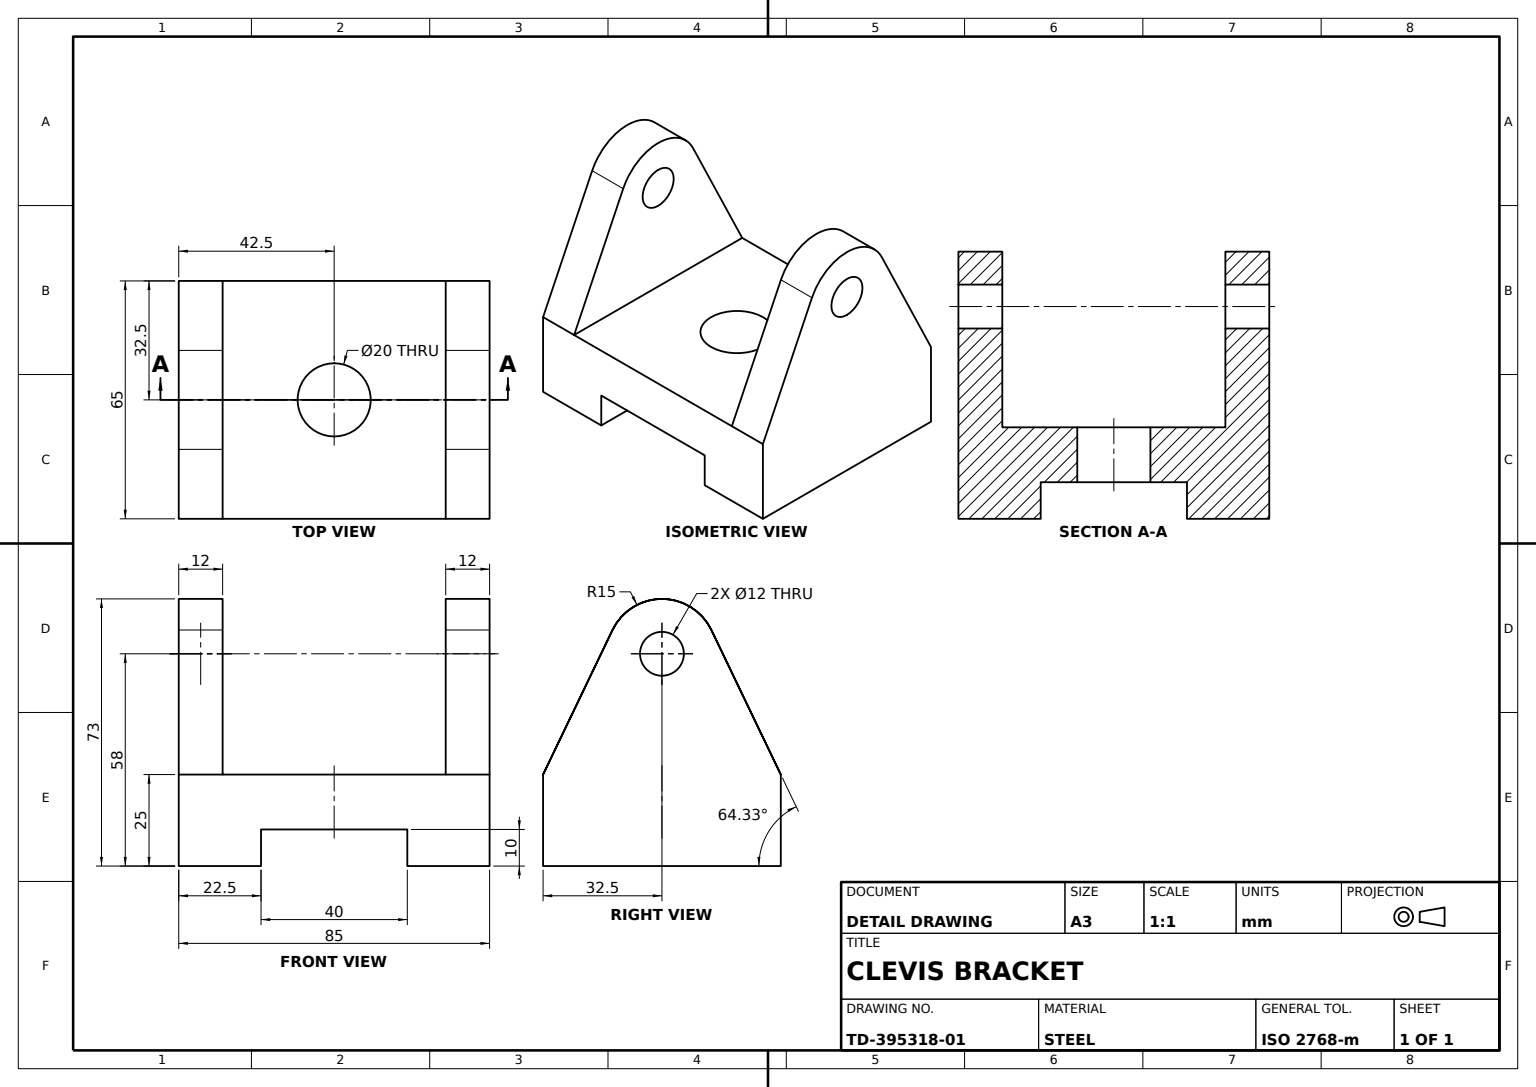
from build123d import *
from build123d.topology import SkipClean

# Parameters (mm, degrees)
BASE_BLOCK_DEPTH     = 32.5
CENTRE_HOLE_SKETCH_R = 10
CENTRE_HOLE_20_DEPTH = 65
LUG_A_BOSS_DEPTH     = 12
LUG_TRIM_CUT_DEPTH   = 102.080413533
LUG_B_BOSS_DEPTH     = 12
PIN_HOLE_SKETCH_R    = 6
PIN_HOLE_CUT_DEPTH   = 102.080413533
LUG_START            = -12
LUG_C_BOSS_DEPTH     = 12
LUG_RIB_A_SKETCH_W   = 61
LUG_RIB_A_SKETCH_H   = 4.481596486
LUG_RIB_A_DEPTH      = 13
LUG_RIB_B_SKETCH_W   = 61
LUG_RIB_B_SKETCH_H   = 4.481596486
LUG_RIB_B_DEPTH      = 13


with BuildPart() as part:
    # Base Profile Sketch → Base Block (new, symmetric)
    with BuildSketch(Plane.XY):
        Polygon((-42.5, 29), (-30.5, 29), (-30.5, -4), (30.5, -4), (30.5, 29), (42.5, 29), (42.5, -29), (20, -29), (20, -19), (-20, -19), (-20, -29), (-42.5, -29), align=None)
    extrude(amount=BASE_BLOCK_DEPTH, both=True)

    # Centre Hole Sketch → Centre Hole Ø20 (cut)
    with BuildSketch(Plane(origin=(0, -4, 0), x_dir=(1, 0, 0), z_dir=(0, 1, 0))):
        with Locations(Location((0, 0, 0), (0, 0, 270))):
            Circle(CENTRE_HOLE_SKETCH_R)
    extrude(amount=-CENTRE_HOLE_20_DEPTH, mode=Mode.SUBTRACT)

    # Lug A Sketch → Lug A Boss (add)
    with BuildSketch(Plane(origin=(42.5, 0, 0), x_dir=(0, 0, -1), z_dir=(1, 0, 0))):
        with BuildLine():
            ThreePointArc((13.519974515, 35.496944598), (0, 44), (-13.519974515, 35.496944598))
            ThreePointArc((-13.519974515, 35.496944598), (-14.625313975, 32.331694935), (-15, 29))
            Line((-15, 29), (-6, 29))
            ThreePointArc((-6, 29), (0, 35), (6, 29))
            Line((6, 29), (15, 29))
            ThreePointArc((15, 29), (14.625313975, 32.331694935), (13.519974515, 35.496944598))
        make_face()
        with BuildLine():
            Line((-6, 29), (-15, 29))
            ThreePointArc((-15, 29), (0, 14), (15, 29))
            Line((15, 29), (6, 29))
            ThreePointArc((6, 29), (0, 23), (-6, 29))
        make_face()
        with BuildLine():
            ThreePointArc((13.519974515, 35.496944598), (0, 44), (-13.519974515, 35.496944598))
            ThreePointArc((-13.519974515, 35.496944598), (-14.625313975, 32.331694935), (-15, 29))
            Line((-15, 29), (-6, 29))
            ThreePointArc((-6, 29), (0, 35), (6, 29))
            Line((6, 29), (15, 29))
            ThreePointArc((15, 29), (14.625313975, 32.331694935), (13.519974515, 35.496944598))
        make_face()
        with BuildLine():
            Line((-6, 29), (-15, 29))
            ThreePointArc((-15, 29), (0, 14), (15, 29))
            Line((15, 29), (6, 29))
            ThreePointArc((6, 29), (0, 23), (-6, 29))
        make_face()
        with BuildLine():
            Line((-16.642043204, 29), (-32.5, -4))
            Line((-32.5, -4), (32.5, -4))
            Line((32.5, -4), (16.642043204, 29))
            Line((16.642043204, 29), (15, 29))
            ThreePointArc((15, 29), (0, 14), (-15, 29))
            Line((-15, 29), (-16.642043204, 29))
        make_face()
        with BuildLine():
            Line((-13.519974515, 35.496944598), (-16.642043204, 29))
            Line((-16.642043204, 29), (-15, 29))
            ThreePointArc((-15, 29), (-14.625313975, 32.331694935), (-13.519974515, 35.496944598))
        make_face()
        with BuildLine():
            Line((15, 29), (16.642043204, 29))
            Line((16.642043204, 29), (13.519974515, 35.496944598))
            ThreePointArc((13.519974515, 35.496944598), (14.625313975, 32.331694935), (15, 29))
        make_face()
    extrude(amount=-LUG_A_BOSS_DEPTH)

    # Lug Trim Sketch → Lug Trim Cut (cut, through all)
    with BuildSketch(Plane(origin=(42.5, 0, 0), x_dir=(0, 0, -1), z_dir=(1, 0, 0))):
        Polygon((-32.5, -17), (-16.642043204, 29), (-32.5, 29), align=None)
        Polygon((32.5, -17), (16.642043204, 29), (32.5, 29), align=None)
    extrude(amount=-LUG_TRIM_CUT_DEPTH, mode=Mode.SUBTRACT)

    # Lug B Sketch → Lug B Boss (add)
    with BuildSketch(Plane(origin=(42.5, 0, 0), x_dir=(0, 0, -1), z_dir=(1, 0, 0))):
        Polygon((-16.642043204, 29), (-32.5, -4), (-32.5, -17), align=None)
        Polygon((32.5, -4), (32.5, -17), (16.642043204, 29), align=None)
    extrude(amount=-LUG_B_BOSS_DEPTH)

    # Pin Hole Sketch → Pin Hole Cut (cut, through all)
    with SkipClean():  # the faces are left unmerged after this step: merging them gives an invalid solid
        with BuildSketch(Plane(origin=(42.5, 0, 0), x_dir=(0, 0, -1), z_dir=(1, 0, 0))):
            with Locations(Location((0, 29, 0), (0, 0, 90))):
                Circle(PIN_HOLE_SKETCH_R)
        extrude(amount=-PIN_HOLE_CUT_DEPTH, mode=Mode.SUBTRACT)

    # Lug C Sketch → Lug C Boss (add)
    with SkipClean():  # the faces are left unmerged after this step: merging them gives an invalid solid
        with BuildSketch(Plane.ZY.offset(42.5).offset(LUG_START)):
            with BuildLine():
                ThreePointArc((13.519974515, 35.496944598), (0, 44), (-13.519974515, 35.496944598))
                ThreePointArc((-13.519974515, 35.496944598), (-14.625313975, 32.331694935), (-15, 29))
                Line((-15, 29), (-6, 29))
                ThreePointArc((-6, 29), (0, 35), (6, 29))
                Line((6, 29), (15, 29))
                ThreePointArc((15, 29), (14.625313975, 32.331694935), (13.519974515, 35.496944598))
            make_face()
            Polygon((-32.5, -4), (-16.642043204, 29), (-32.5, -17), align=None)
            Polygon((32.5, -17), (32.5, -4), (16.642043204, 29), align=None)
            with BuildLine():
                Line((-13.519974515, 35.496944598), (-16.642043204, 29))
                Line((-16.642043204, 29), (-15, 29))
                ThreePointArc((-15, 29), (-14.625313975, 32.331694935), (-13.519974515, 35.496944598))
            make_face()
            with BuildLine():
                Line((16.642043204, 29), (13.519974515, 35.496944598))
                ThreePointArc((13.519974515, 35.496944598), (14.625313975, 32.331694935), (15, 29))
                Line((15, 29), (16.642043204, 29))
            make_face()
        extrude(amount=LUG_C_BOSS_DEPTH)

    # Lug Rib A Sketch → Lug Rib A (add)
    with SkipClean():  # the faces are left unmerged after this step: merging them gives an invalid solid
        with BuildSketch(Plane(origin=(0, -4, 0), x_dir=(1, 0, 0), z_dir=(0, 1, 0))):
            with Locations((0, 30.259201757)):
                Rectangle(LUG_RIB_A_SKETCH_W, LUG_RIB_A_SKETCH_H)
        extrude(amount=-LUG_RIB_A_DEPTH)

    # Lug Rib B Sketch → Lug Rib B (add)
    with SkipClean():  # the faces are left unmerged after this step: merging them gives an invalid solid
        with BuildSketch(Plane(origin=(0, -4, 0), x_dir=(1, 0, 0), z_dir=(0, 1, 0))):
            with Locations((0, -30.259201757)):
                Rectangle(LUG_RIB_B_SKETCH_W, LUG_RIB_B_SKETCH_H)
        extrude(amount=-LUG_RIB_B_DEPTH)


solid = part.part
